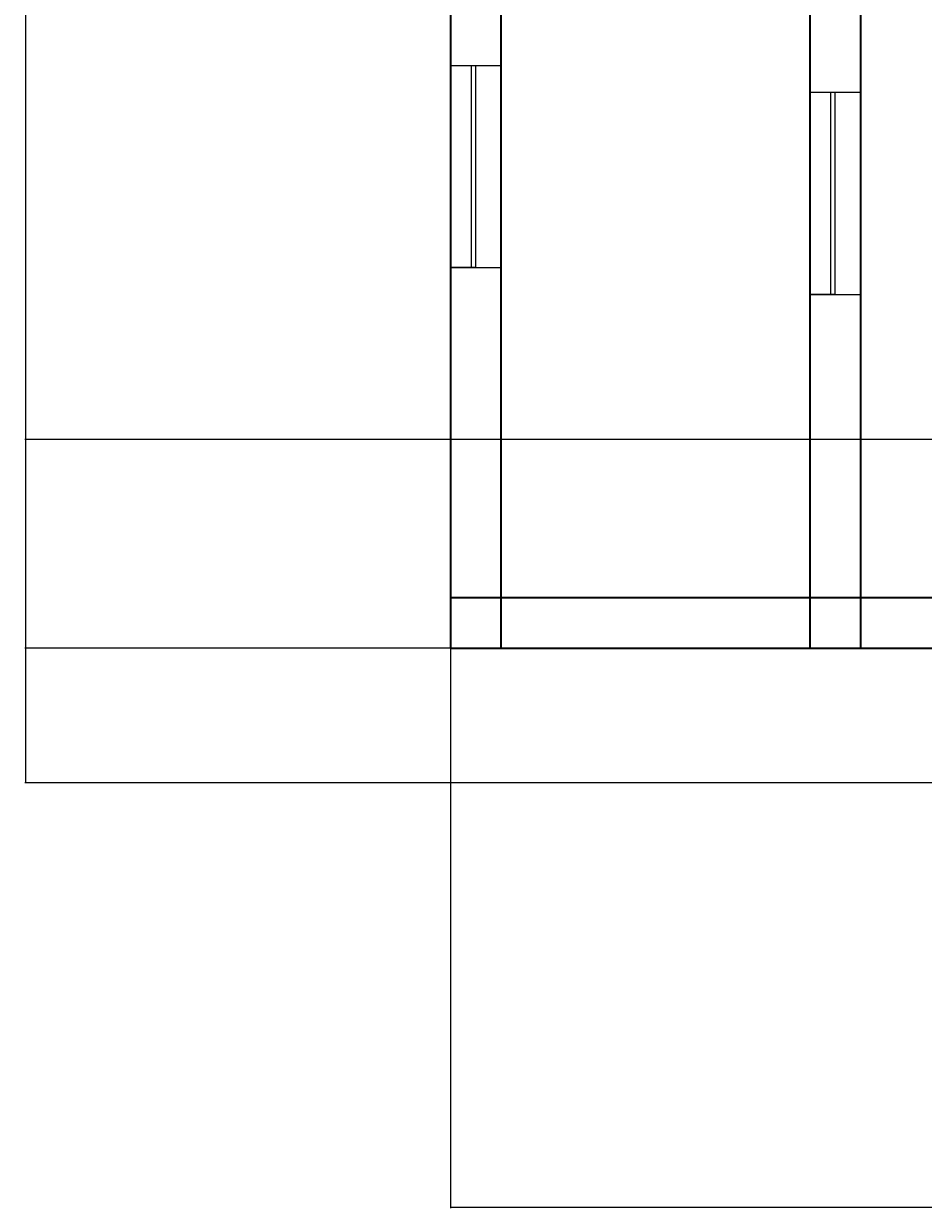
# Model space of a CAD drawing. Units: inches. Extents: x -61 to 1599, y -1316 to 257.
# Tile 1 of 204: x -61 to 99, y -1316 to -1105. Entities that reach past the tile are written whole.
import ezdxf

# ---------------------------------------------------------------- set-up
doc = ezdxf.new("R2010")
doc.units = ezdxf.units.IN
doc.header["$MEASUREMENT"] = 0
for name, color, linetype, lineweight in [('A-ANNO-DIMS', 2, 'Continuous', 18), ('WALLS', 4, 'Continuous', 35), ('WINDOWS', 220, 'Continuous', 18)]:
    doc.layers.add(name, color=color, linetype=linetype, lineweight=lineweight)
doc.styles.get("Standard").update_dxf_attribs({"font": 'arial.ttf'})
doc.dimstyles.get("Standard").update_dxf_attribs({"dimtxt": 0.18, "dimasz": 0.18, "dimexe": 0.18, "dimexo": 0.0625, "dimgap": 0.09, "dimtad": 0, "dimtih": 1, "dimtoh": 1, "dimdec": 0, "dimzin": 0, "dimdsep": 46, "dimlunit": 3, "dimtxsty": 'Standard', "dimcen": 0.09, "dimadec": 0, "dimazin": 0, "dimtfac": 1, "dimtdec": 0, "dimtofl": 0, "dimtmove": 0, "dimatfit": 3, "dimfxl": 1, "dimtolj": 1, "dimtzin": 0, "dimarcsym": 0})

# ---------------------------------------------------------------- blocks, each defined once
blk = doc.blocks.new('WIN-36IN')
for p, q in [((0, 4.5), (0, 9)), ((0, 9), (0, 0)), ((36, 9), (36, 0)), ((0, 5.26), (36, 5.26)), ((0, 4.5), (36, 4.5)), ((0, 4.5), (36, 4.5))]:
    blk.add_line(p, q)
blk = doc.blocks.new('*D687')
at = {"layer": 'A-ANNO-DIMS', "color": 0, "lineweight": -2, "transparency": 16777216}
for p, q in [((289.42, 181.68), (-61.08, 181.68)), ((-60.9, 181.5), (-60.9, -528.95)), ((-60.9, -1239.76), (-60.9, -529.32)), ((319.64, -1239.94), (-61.08, -1239.94))]:
    blk.add_line(p, q, dxfattribs=at)
at = {"layer": 'A-ANNO-DIMS', "color": 0, "transparency": 16777216}
for points in [[(-60.93, 181.5), (-60.87, 181.5), (-60.9, 181.68)], [(-60.93, -1239.76), (-60.87, -1239.76), (-60.9, -1239.94)]]:
    blk.add_solid(points, dxfattribs=at)
at = {"layer": 'DEFPOINTS', "color": 0, "transparency": 16777216}
for p in [(289.48, 181.68), (-60.9, -1239.94), (319.7, -1239.94)]:
    blk.add_point(p, dxfattribs=at)
at = {"layer": 'A-ANNO-DIMS', "color": 0, "transparency": 16777216, "insert": (-60.9, -529.13), "char_height": 0.18, "attachment_point": 5}
blk.add_mtext('\\A1;1421.6', dxfattribs=at)
blk = doc.blocks.new('*D688')
at = {"layer": 'A-ANNO-DIMS', "color": 0, "lineweight": -2, "transparency": 16777216}
for p, q in [((14.7, -1216.01), (14.7, -1315.72)), ((544.7, -1216.01), (544.7, -1315.72)), ((14.88, -1315.54), (279.41, -1315.54)), ((544.52, -1315.54), (279.99, -1315.54))]:
    blk.add_line(p, q, dxfattribs=at)
at = {"layer": 'A-ANNO-DIMS', "color": 0, "transparency": 16777216}
for points in [[(14.88, -1315.51), (14.88, -1315.57), (14.7, -1315.54)], [(544.52, -1315.51), (544.52, -1315.57), (544.7, -1315.54)]]:
    blk.add_solid(points, dxfattribs=at)
at = {"layer": 'DEFPOINTS', "color": 0, "transparency": 16777216}
for p in [(14.7, -1215.94), (544.7, -1215.94), (544.7, -1315.54)]:
    blk.add_point(p, dxfattribs=at)
at = {"layer": 'A-ANNO-DIMS', "color": 0, "transparency": 16777216, "insert": (279.7, -1315.54), "char_height": 0.18, "attachment_point": 5}
blk.add_mtext('\\A1;530', dxfattribs=at)
blk = doc.blocks.new('*D693')
at = {"layer": 'A-ANNO-DIMS', "color": 0, "lineweight": -2, "transparency": 16777216}
for p, q in [((14.64, -616.94), (-61.08, -616.94)), ((-60.9, -617.12), (-60.9, -916.26)), ((-60.9, -1215.76), (-60.9, -916.63)), ((14.64, -1215.94), (-61.08, -1215.94))]:
    blk.add_line(p, q, dxfattribs=at)
at = {"layer": 'A-ANNO-DIMS', "color": 0, "transparency": 16777216}
for points in [[(-60.93, -617.12), (-60.87, -617.12), (-60.9, -616.94)], [(-60.93, -1215.76), (-60.87, -1215.76), (-60.9, -1215.94)]]:
    blk.add_solid(points, dxfattribs=at)
at = {"layer": 'DEFPOINTS', "color": 0, "transparency": 16777216}
for p in [(-60.9, -616.94), (14.7, -616.94), (14.7, -1215.94)]:
    blk.add_point(p, dxfattribs=at)
at = {"layer": 'A-ANNO-DIMS', "color": 0, "transparency": 16777216, "insert": (-60.9, -916.44), "char_height": 0.18, "attachment_point": 5}
blk.add_mtext('\\A1;599', dxfattribs=at)
blk = doc.blocks.new('*D696')
at = {"layer": 'A-ANNO-DIMS', "color": 0, "lineweight": -2, "transparency": 16777216}
for p, q in [((690.64, -873.17), (-61.08, -873.17)), ((-60.9, -873.35), (-60.9, -1025.8)), ((-60.9, -1178.61), (-60.9, -1026.16)), ((690.64, -1178.79), (-61.08, -1178.79))]:
    blk.add_line(p, q, dxfattribs=at)
at = {"layer": 'A-ANNO-DIMS', "color": 0, "transparency": 16777216}
for points in [[(-60.93, -873.35), (-60.87, -873.35), (-60.9, -873.17)], [(-60.93, -1178.61), (-60.87, -1178.61), (-60.9, -1178.79)]]:
    blk.add_solid(points, dxfattribs=at)
at = {"layer": 'DEFPOINTS', "color": 0, "transparency": 16777216}
for p in [(-60.9, -873.17), (690.7, -873.17), (690.7, -1178.79)]:
    blk.add_point(p, dxfattribs=at)
at = {"layer": 'A-ANNO-DIMS', "color": 0, "transparency": 16777216, "insert": (-60.9, -1025.98), "char_height": 0.18, "attachment_point": 5}
blk.add_mtext('\\A1;305.6', dxfattribs=at)

msp = doc.modelspace()

# ---------------------------------------------------------------- linework, layer by layer
at = {"layer": 'WALLS'}
for p, q in [((14.7028, -616.9446), (14.7028, -1215.9446)), ((23.7028, -943.9446), (23.7028, -1215.9446)), ((78.7028, -943.9446), (78.7028, -1215.9446)), ((87.7028, -1056.9446), (87.7028, -1215.9446)), ((14.7028, -1206.9446), (237.7028, -1206.9446)), ((14.7028, -1215.9446), (237.7028, -1215.9446))]:
    msp.add_line(p, q, dxfattribs=at)

# ---------------------------------------------------------------- block references
at = {"layer": 'WINDOWS'}
for p, rotation in [((23.7029, -1148.1651), 90.00000000000017), ((87.7029, -1152.9406), 90.00000000000006)]:
    msp.add_blockref('WIN-36IN', p, dxfattribs=dict(at, rotation=rotation))

# ---------------------------------------------------------------- dimensions: what is measured, and where the dimension line sits
at = {"layer": 'A-ANNO-DIMS'}
for base, p1, p2, override, picture, middle in [((-60.8972, -1239.9446), (289.4807, 181.6771), (319.7028, -1239.9446), {"dimdec": 1, "dimlfac": 1, "dimrnd": 0, "dimzin": 0, "dimdsep": 46, "dimlunit": 2}, '*D687', (-60.8972, -529.1337)), ((-60.8972, -616.9446), (14.7028, -1215.9446), (14.7028, -616.9446), {"dimdec": 0, "dimlfac": 1, "dimrnd": 0, "dimzin": 0, "dimdsep": 46, "dimlunit": 2}, '*D693', (-60.8972, -916.4446)), ((-60.8972, -873.169), (690.7028, -1178.7933), (690.7028, -873.169), {"dimdec": 1, "dimlfac": 1, "dimrnd": 0, "dimzin": 0, "dimdsep": 46, "dimlunit": 2}, '*D696', (-60.8972, -1025.9812))]:
    dim = msp.add_linear_dim(base=base, p1=p1, p2=p2, angle=90, dimstyle='Standard', override=override, dxfattribs=at)
    dim.commit()
    dim.dimension.update_dxf_attribs({"geometry": picture, "text_midpoint": middle})
dim = msp.add_linear_dim(base=(544.7028, -1315.5446), p1=(14.7028, -1215.9446), p2=(544.7028, -1215.9446), dimstyle='Standard', override={"dimdec": 0, "dimlfac": 1, "dimrnd": 0, "dimzin": 0, "dimdsep": 46, "dimlunit": 2}, dxfattribs=at)
dim.commit()
dim.dimension.update_dxf_attribs({"geometry": '*D688', "text_midpoint": (279.7028, -1315.5446)})

doc.saveas('drawing.dxf')
